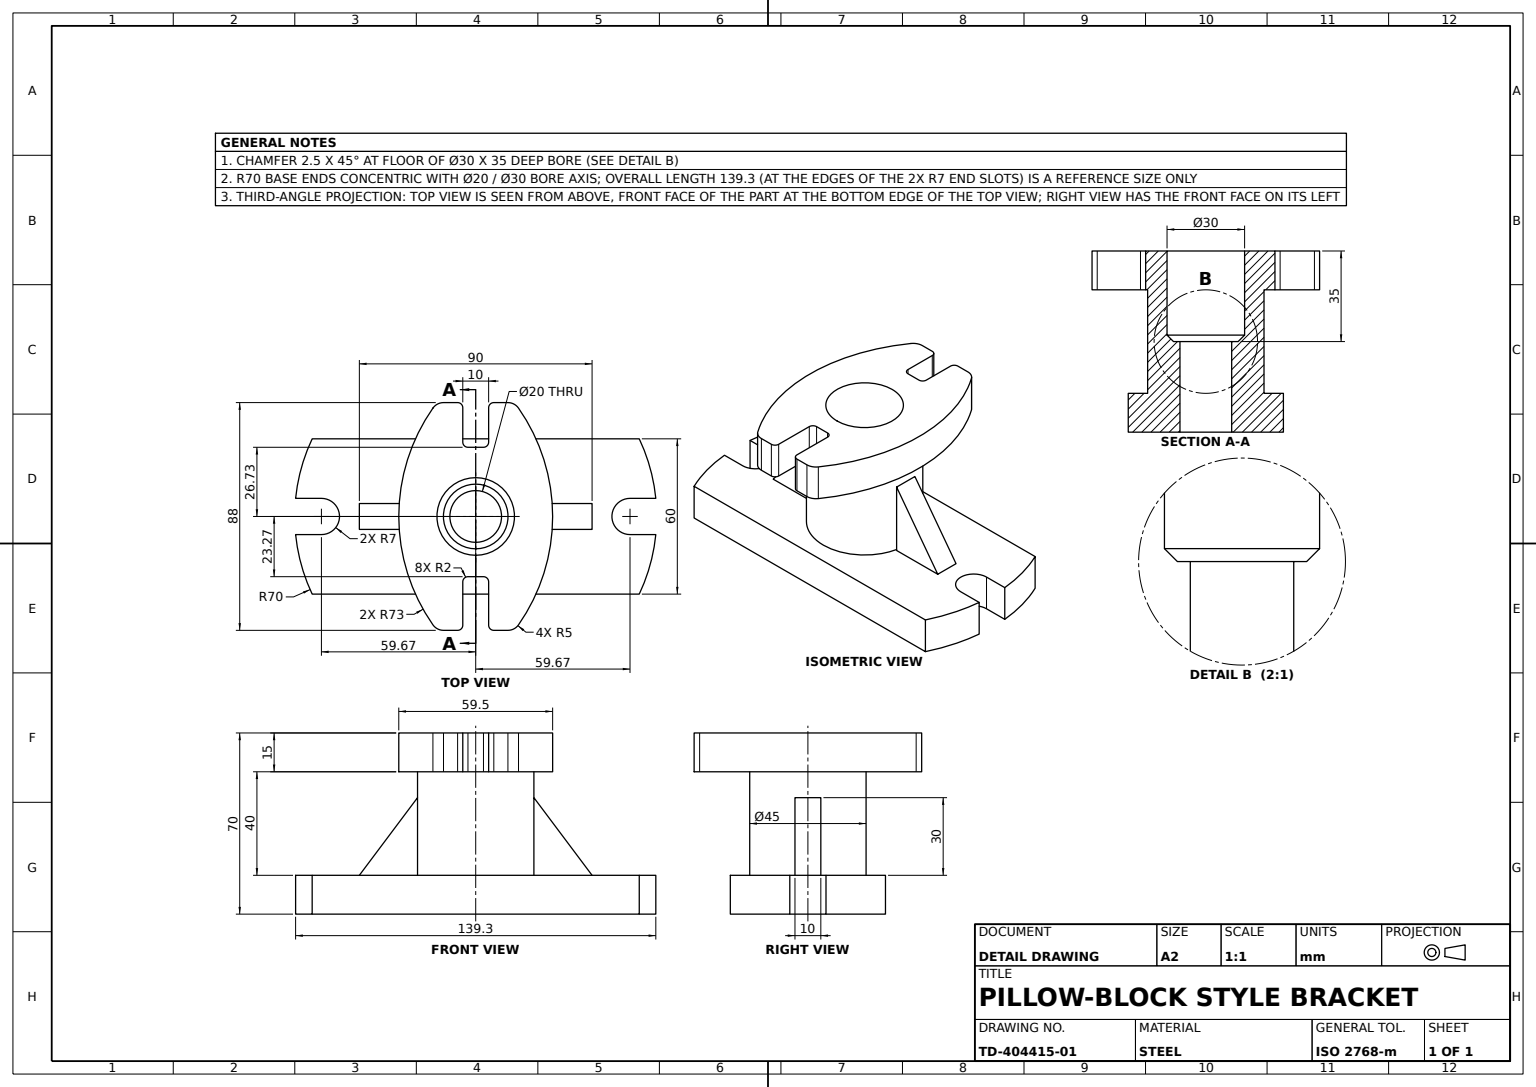
SolidWorks part; units mm, degrees
material "Plain Carbon Steel"
ref_plane "Front Plane" through (0, 0, 0) normal (0, 0, 1) x (1, 0, 0)
ref_plane "Top Plane" through (0, 0, 0) normal (0, 1, 0) x (1, 0, 0)
ref_plane "Right Plane" through (0, 0, 0) normal (1, 0, 0) x (0, 0, -1)
sketch "Base Plate Sketch" plane through (0, 0, 0) normal (0, 1, 0) x (1, 0, 0)
  line L0 (0, 44.7146) -> (0, -49.9154) construction
  line L1 (72.3044, 0) -> (-84.7357, 0) construction
  line L2 (-69.6491, 7) -> (-59.6693, 7)
  line L3 (-63.2456, 30) -> (63.2456, 30)
  line L5 (-63.2456, -30) -> (63.2456, -30)
  line L7 (-69.6491, -7) -> (-59.6693, -7)
  line L8 (69.6491, -7) -> (59.6693, -7)
  line L9 (69.6491, 7) -> (59.6693, 7)
  arc A0 (-69.6491, -7) -> (-63.2456, -30) centre (0, 0) ccw
  arc A1 (-59.6693, -7) -> (-59.6693, 7) centre (-59.6693, 0) ccw
  arc A3 (-63.2456, 30) -> (-69.6491, 7) centre (0, 0) ccw
  arc A4 (63.2456, -30) -> (69.6491, -7) centre (0, 0) ccw
  arc A5 (59.6693, -7) -> (59.6693, 7) centre (59.6693, 0) cw
  arc A6 (69.6491, 7) -> (63.2456, 30) centre (0, 0) ccw
  point P5 (0, 0)
  dimension "D3" = 140
  dimension "D4" = 14
  dimension "D1" = 59.6693
  dimension "D2" = 60
extrude "Base Plate" add sketch "Base Plate Sketch" along normal blind 15
sketch "Boss Sketch Ø45" plane through (0, 15, 0) normal (0, 1, 0) x (1, 0, 0)
  circle A0 centre (0, 0) radius 22.5
  dimension "D1" = 45
extrude "Boss Ø45" add sketch "Boss Sketch Ø45" along normal blind 40
sketch "Top Flange Sketch" plane through (0, 55, 0) normal (0, 1, 0) x (1, 0, 0)
  line L0 (7, -44) -> (15, -44)
  line L1 (-15, 44) -> (-7, 44)
  line L3 (-15, -44) -> (-7, -44)
  line L5 (0, -62.7538) -> (0, 65.7744) construction
  line L8 (-5, 42) -> (-5, 25.2669)
  line L9 (-3, 23.2669) -> (3, 23.2669)
  line L10 (5, 42) -> (5, 25.2669)
  line L14 (-5, -42) -> (-5, -28.7331)
  line L15 (-3, -26.7331) -> (3, -26.7331)
  line L16 (5, -42) -> (5, -28.7331)
  line L19 (7, 44) -> (15, 44)
  arc A0 (-15, 44) -> (-15, -44) centre (43.2495, 0) ccw
  arc A1 (3, -26.7331) -> (5, -28.7331) centre (3, -28.7331) cw
  circle A2 centre (0, 0) radius 22.5 construction
  arc A3 (15, 44) -> (15, -44) centre (-43.2495, 0) cw
  arc A4 (-3, -26.7331) -> (-5, -28.7331) centre (-3, -28.7331) ccw
  arc A5 (3, 23.2669) -> (5, 25.2669) centre (3, 25.2669) ccw
  arc A6 (-3, 23.2669) -> (-5, 25.2669) centre (-3, 25.2669) cw
  arc A7 (5, -42) -> (7, -44) centre (7, -42) ccw
  arc A8 (-7, -44) -> (-5, -42) centre (-7, -42) ccw
  arc A9 (5, 42) -> (7, 44) centre (7, 42) cw
  arc A10 (-5, 42) -> (-7, 44) centre (-7, 42) ccw
  point P0 (0, 0)
  point P22 (5, -26.7331)
  point P25 (-5, -26.7331)
  point P28 (5, 23.2669)
  point P31 (-5, 23.2669)
  point P34 (5, -44)
  point P37 (-5, -44)
  point P40 (5, 44)
  dimension "D3" = 146
  dimension "D8" = 2
  dimension "D9" = 2
  dimension "D1" = 88
  dimension "D2" = 30
  dimension "D4" = 5
  dimension "D5" = 44
  dimension "D6" = 23.2669
  dimension "D7" = 26.7331
extrude "Top Flange" add sketch "Top Flange Sketch" along normal blind 15
sketch "Counterbore Sketch Ø30" plane through (0, 70, 0) normal (0, 1, 0) x (1, 0, 0)
  circle A0 centre (0, 0) radius 15
  dimension "D1" = 30
extrude "Counterbore Ø30" cut sketch "Counterbore Sketch Ø30" against normal blind 35
sketch "Through Bore Sketch Ø20" plane through (0, 35, 0) normal (0, 1, 0) x (1, 0, 0)
  circle A0 centre (0, 0) radius 10
  dimension "D1" = 20
extrude "Through Bore Ø20" cut sketch "Through Bore Sketch Ø20" against normal blind 35
chamfer "Bore Chamfer 2.5" distance 2.5 angle 45 1 edges at (0, 35, 15)
sketch "Gusset Rib Sketch" plane through (0, 0, 0) normal (0, 0, 1) x (1, 0, 0)
  line L0 (-22.5, 55) -> (-22.5, 15) construction
  line L1 (-22.5, 45) -> (-22.5, 15)
  line L2 (-63.2456, 15) -> (63.2456, 15) construction
  line L3 (-45, 15) -> (-22.5, 15)
  line L4 (-22.5, 45) -> (-45, 15)
  line L5 (0, 48.8701) -> (0, -14.3136) construction
  dimension "D1" = 30
  dimension "D2" = 45
extrude "Gusset Rib" add sketch "Gusset Rib Sketch" along normal mid plane 10 separate body
mirror "Gusset Rib Mirror" about plane through (0, 0, 0) normal (1, 0, 0) of bodies 108
fillet "Flange Fillets R5" radius 5 4 edges at (15, 62.5, -44) (-15, 62.5, -44) (15, 62.5, 44) (-15, 62.5, 44)
